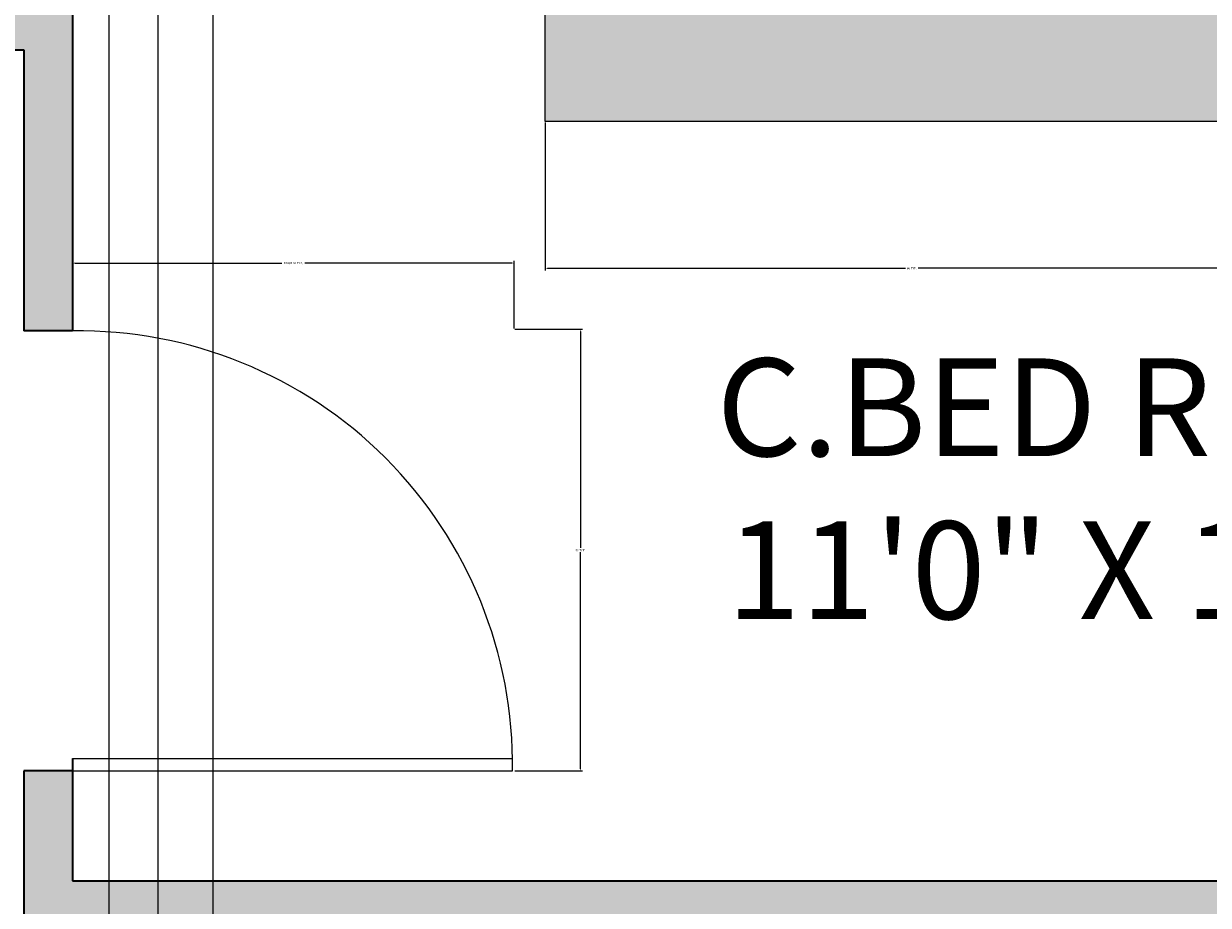
# Model space of a CAD drawing. Units: inches. Extents: x 1567 to 1964, y 1813 to 2447.
# Tile 25 of 28: x 1788 to 1885, y 2261 to 2333. Entities that reach past the tile are written whole.
import ezdxf

# ---------------------------------------------------------------- set-up
doc = ezdxf.new("R2010")
doc.units = ezdxf.units.IN
for name, color, linetype, lineweight in [('A-ANNO-DIMS', 2, 'Continuous', 18), ('A-AREA-IDEN', 7, 'Continuous', 18), ('A-DOOR', 4, 'Continuous', 18), ('A-FURN', 8, 'Continuous', 18), ('A-WALL', 7, 'Continuous', 35)]:
    doc.layers.add(name, color=color, linetype=linetype, lineweight=lineweight)
doc.layers.add('A-FURN-PATT', color=252, linetype='Continuous', lineweight=13, true_color=0x939598)
doc.layers.add('A-WALL-PATT', color=251, linetype='Continuous', lineweight=13, true_color=0x636466)
doc.styles.get("Standard").update_dxf_attribs({"font": 'arial.ttf'})
doc.dimstyles.get("Standard").update_dxf_attribs({"dimtxt": 0.18, "dimasz": 0.18, "dimexe": 0.18, "dimexo": 0.0625, "dimgap": 0.09, "dimtad": 0, "dimtih": 1, "dimtoh": 1, "dimdec": 4, "dimzin": 0, "dimdsep": 46, "dimtxsty": 'Standard', "dimcen": 0.09, "dimadec": 0, "dimazin": 0, "dimtfac": 1, "dimtdec": 4, "dimtofl": 0, "dimtmove": 0, "dimatfit": 3, "dimfxl": 1, "dimtolj": 1, "dimtzin": 0, "dimarcsym": 0})

# ---------------------------------------------------------------- blocks, each defined once
blk = doc.blocks.new('Bed - Queen')
for p, q in [((0, -80.00003), (0, 0)), ((59.99999, -80.00003), (0, -80.00003))]:
    blk.add_line(p, q)
blk = doc.blocks.new('DOOR-SWING-36IN')
for p, q in [((0, 36.001), (0, 0.001)), ((1, 36.001), (1, 0.001))]:
    blk.add_line(p, q)
blk.add_arc((0.5, 35.501), 35.504, 269.19307, 0.80693)
blk = doc.blocks.new('*D16')
at = {"layer": 'A-ANNO-DIMS', "color": 0, "lineweight": -2, "transparency": 16777216}
for p, q in [((1831.109, 2325.358), (1831.109, 2313.24)), ((1891.109, 2325.358), (1891.109, 2313.24)), ((1831.289, 2313.42), (1860.581, 2313.42)), ((1890.929, 2313.42), (1861.638, 2313.42))]:
    blk.add_line(p, q, dxfattribs=at)
at = {"layer": 'A-ANNO-DIMS', "color": 0, "transparency": 16777216}
for points in [[(1831.289, 2313.45), (1831.289, 2313.39), (1831.109, 2313.42)], [(1890.929, 2313.45), (1890.929, 2313.39), (1891.109, 2313.42)]]:
    blk.add_solid(points, dxfattribs=at)
at = {"layer": 'Defpoints', "color": 0, "transparency": 16777216}
for p in [(1831.109, 2325.42), (1891.109, 2325.42), (1891.109, 2313.42)]:
    blk.add_point(p, dxfattribs=at)
at = {"layer": 'A-ANNO-DIMS', "color": 0, "transparency": 16777216, "insert": (1861.109, 2313.42), "char_height": 0.18, "attachment_point": 5}
blk.add_mtext('\\A1;60 TYP.', dxfattribs=at)
blk = doc.blocks.new('*D29')
at = {"layer": 'A-ANNO-DIMS', "color": 0, "lineweight": -2, "transparency": 16777216}
for p, q in [((1792.43, 2308.488), (1792.43, 2314.025)), ((1828.565, 2308.488), (1828.565, 2314.025)), ((1792.61, 2313.845), (1809.561, 2313.845)), ((1828.385, 2313.845), (1811.433, 2313.845))]:
    blk.add_line(p, q, dxfattribs=at)
at = {"layer": 'A-ANNO-DIMS', "color": 0, "transparency": 16777216}
for points in [[(1792.61, 2313.875), (1792.61, 2313.815), (1792.43, 2313.845)], [(1828.385, 2313.875), (1828.385, 2313.815), (1828.565, 2313.845)]]:
    blk.add_solid(points, dxfattribs=at)
at = {"layer": 'Defpoints', "color": 0, "transparency": 16777216}
for p in [(1792.43, 2313.845), (1792.43, 2308.425), (1828.565, 2308.425)]:
    blk.add_point(p, dxfattribs=at)
at = {"layer": 'A-ANNO-DIMS', "color": 0, "transparency": 16777216, "insert": (1810.497, 2313.845), "char_height": 0.18, "attachment_point": 5}
blk.add_mtext('\\A1;DOOR 36 TYP.', dxfattribs=at)
blk = doc.blocks.new('*D30')
at = {"layer": 'A-ANNO-DIMS', "color": 0, "lineweight": -2, "transparency": 16777216}
for p, q in [((1828.627, 2308.425), (1834.165, 2308.425)), ((1833.985, 2308.245), (1833.985, 2290.539)), ((1833.985, 2272.47), (1833.985, 2290.176)), ((1828.627, 2272.29), (1834.165, 2272.29))]:
    blk.add_line(p, q, dxfattribs=at)
at = {"layer": 'A-ANNO-DIMS', "color": 0, "transparency": 16777216}
for points in [[(1833.955, 2308.245), (1834.015, 2308.245), (1833.985, 2308.425)], [(1833.955, 2272.47), (1834.015, 2272.47), (1833.985, 2272.29)]]:
    blk.add_solid(points, dxfattribs=at)
at = {"layer": 'Defpoints', "color": 0, "transparency": 16777216}
for p in [(1828.565, 2308.425), (1833.985, 2308.425), (1828.565, 2272.29)]:
    blk.add_point(p, dxfattribs=at)
at = {"layer": 'A-ANNO-DIMS', "color": 0, "transparency": 16777216, "insert": (1833.985, 2290.358), "char_height": 0.18, "attachment_point": 5}
blk.add_mtext('\\A1;36 TYP.', dxfattribs=at)
blk = doc.blocks.new('*D54')
at = {"layer": 'A-ANNO-DIMS', "color": 0, "lineweight": -2, "transparency": 16777216}
for p, q in [((1711.43, 1964.352), (1711.43, 2447.12)), ((1711.61, 2446.94), (1753.211, 2446.94)), ((1795.25, 2446.94), (1753.648, 2446.94)), ((1795.43, 1964.352), (1795.43, 2447.12))]:
    blk.add_line(p, q, dxfattribs=at)
at = {"layer": 'A-ANNO-DIMS', "color": 0, "transparency": 16777216}
for points in [[(1711.61, 2446.97), (1711.61, 2446.91), (1711.43, 2446.94)], [(1795.25, 2446.97), (1795.25, 2446.91), (1795.43, 2446.94)]]:
    blk.add_solid(points, dxfattribs=at)
at = {"layer": 'Defpoints', "color": 0, "transparency": 16777216}
for p in [(1795.43, 2446.94), (1711.43, 1964.29), (1795.43, 1964.29)]:
    blk.add_point(p, dxfattribs=at)
at = {"layer": 'A-ANNO-DIMS', "color": 0, "transparency": 16777216, "insert": (1753.43, 2446.94), "char_height": 0.18, "attachment_point": 5}
blk.add_mtext('\\A1;84', dxfattribs=at)
blk = doc.blocks.new('*D55')
at = {"layer": 'A-ANNO-DIMS', "color": 0, "lineweight": -2, "transparency": 16777216}
for p, q in [((1795.43, 1964.352), (1795.43, 2447.12)), ((1795.61, 2446.94), (1797.277, 2446.94)), ((1799.25, 2446.94), (1797.582, 2446.94)), ((1799.43, 1967.352), (1799.43, 2447.12))]:
    blk.add_line(p, q, dxfattribs=at)
at = {"layer": 'A-ANNO-DIMS', "color": 0, "transparency": 16777216}
for points in [[(1795.61, 2446.97), (1795.61, 2446.91), (1795.43, 2446.94)], [(1799.25, 2446.97), (1799.25, 2446.91), (1799.43, 2446.94)]]:
    blk.add_solid(points, dxfattribs=at)
at = {"layer": 'Defpoints', "color": 0, "transparency": 16777216}
for p in [(1799.43, 2446.94), (1799.43, 1967.29), (1795.43, 1964.29)]:
    blk.add_point(p, dxfattribs=at)
at = {"layer": 'A-ANNO-DIMS', "color": 0, "transparency": 16777216, "insert": (1797.43, 2446.94), "char_height": 0.18, "attachment_point": 5}
blk.add_mtext('\\A1;4', dxfattribs=at)
blk = doc.blocks.new('*D70')
at = {"layer": 'A-ANNO-DIMS', "color": 0, "lineweight": -2, "transparency": 16777216}
for p, q in [((1799.43, 1967.352), (1799.43, 2447.12)), ((1799.61, 2446.94), (1801.421, 2446.94)), ((1803.75, 2446.94), (1801.938, 2446.94)), ((1803.93, 1967.352), (1803.93, 2447.12))]:
    blk.add_line(p, q, dxfattribs=at)
at = {"layer": 'A-ANNO-DIMS', "color": 0, "transparency": 16777216}
for points in [[(1799.61, 2446.97), (1799.61, 2446.91), (1799.43, 2446.94)], [(1803.75, 2446.97), (1803.75, 2446.91), (1803.93, 2446.94)]]:
    blk.add_solid(points, dxfattribs=at)
at = {"layer": 'Defpoints', "color": 0, "transparency": 16777216}
for p in [(1803.93, 2446.94), (1799.43, 1967.29), (1803.93, 1967.29)]:
    blk.add_point(p, dxfattribs=at)
at = {"layer": 'A-ANNO-DIMS', "color": 0, "transparency": 16777216, "insert": (1801.68, 2446.94), "char_height": 0.18, "attachment_point": 5}
blk.add_mtext('\\A1;4.5', dxfattribs=at)
blk = doc.blocks.new('*D71')
at = {"layer": 'A-ANNO-DIMS', "color": 0, "lineweight": -2, "transparency": 16777216}
for p, q in [((1799.43, 1910.752), (1799.43, 2447.12)), ((1799.61, 2446.94), (1861.648, 2446.94)), ((1924.25, 2446.94), (1862.211, 2446.94)), ((1924.43, 1910.752), (1924.43, 2447.12))]:
    blk.add_line(p, q, dxfattribs=at)
at = {"layer": 'A-ANNO-DIMS', "color": 0, "transparency": 16777216}
for points in [[(1799.61, 2446.97), (1799.61, 2446.91), (1799.43, 2446.94)], [(1924.25, 2446.97), (1924.25, 2446.91), (1924.43, 2446.94)]]:
    blk.add_solid(points, dxfattribs=at)
at = {"layer": 'Defpoints', "color": 0, "transparency": 16777216}
for p in [(1924.43, 2446.94), (1799.43, 1910.69), (1924.43, 1910.69)]:
    blk.add_point(p, dxfattribs=at)
at = {"layer": 'A-ANNO-DIMS', "color": 0, "transparency": 16777216, "insert": (1861.93, 2446.94), "char_height": 0.18, "attachment_point": 5}
blk.add_mtext('\\A1;125', dxfattribs=at)

msp = doc.modelspace()

# ---------------------------------------------------------------- hatches: boundary and pattern name
at = {"layer": 'A-FURN-PATT'}
h = msp.add_hatch(color=256, dxfattribs=at)
h.dxf.hatch_style = 1
h.paths.add_polyline_path([(1697.3402, 2374.8316), (1682.1402, 2374.8316), (1682.1402, 2387.6316), (1637.3402, 2387.6316), (1637.3402, 2324.4315), (1697.3402, 2324.4315)])
h.paths.add_polyline_path([(1891.1093, 2375.8204), (1875.9094, 2375.8204), (1875.9094, 2388.6204), (1831.1094, 2388.6204), (1831.1094, 2325.4204), (1891.1093, 2325.4204)])
h.paths.add_polyline_path([(1702.5611, 2206.8057), (1702.5611, 2210.8057), (1699.7395, 2209.9436), (1697.013, 2209.2403), (1694.3857, 2208.6763), (1691.8615, 2208.2326), (1689.4443, 2207.8896), (1687.1381, 2207.6282), (1684.9469, 2207.4289), (1682.8747, 2207.2725), (1680.9233, 2207.1425), (1679.0865, 2207.0339), (1677.3558, 2206.9445), (1675.7229, 2206.8719), (1674.1794, 2206.8141), (1672.7169, 2206.7688), (1671.327, 2206.7339), (1670.0014, 2206.707), (1668.7314, 2206.6866), (1667.5072, 2206.6732), (1666.3188, 2206.668), (1665.1561, 2206.6722), (1664.009, 2206.6869), (1662.8675, 2206.7133), (1661.7215, 2206.7525), (1660.5611, 2206.8057), (1660.5611, 2202.8057), (1661.9932, 2202.9556), (1663.3314, 2203.0744), (1664.5899, 2203.1671), (1665.7831, 2203.2385), (1666.9254, 2203.2935), (1668.0311, 2203.3368), (1669.1145, 2203.3734), (1670.1902, 2203.4081), (1671.2724, 2203.4451), (1672.3759, 2203.4866), (1673.5155, 2203.534), (1674.706, 2203.5887), (1675.9621, 2203.6523), (1677.2986, 2203.7262), (1678.7304, 2203.8118), (1680.2722, 2203.9108), (1681.947, 2204.0272), (1683.8108, 2204.1769), (1685.9279, 2204.3782), (1688.3626, 2204.6496), (1691.179, 2205.0096), (1694.4413, 2205.4767), (1698.214, 2206.0692)])
h.paths.add_polyline_path([(1702.5611, 2218.8057), (1701.9821, 2217.9383), (1701.3316, 2217.191), (1700.6091, 2216.5515), (1699.8141, 2216.0071), (1698.946, 2215.5454), (1698.0041, 2215.1536), (1696.9879, 2214.8194), (1695.8969, 2214.5301), (1694.7328, 2214.2753), (1693.5072, 2214.0522), (1692.2339, 2213.8602), (1690.9266, 2213.6989), (1689.5994, 2213.5675), (1688.266, 2213.4654), (1686.9402, 2213.392), (1685.636, 2213.3467), (1684.3619, 2213.3287), (1683.1053, 2213.3361), (1681.8482, 2213.3668), (1680.5727, 2213.4187), (1679.2608, 2213.4898), (1677.8948, 2213.5779), (1676.4565, 2213.6811), (1674.9282, 2213.7971), (1673.2982, 2213.9236), (1671.5804, 2214.0573), (1669.795, 2214.1945), (1667.9622, 2214.3316), (1666.1022, 2214.4649), (1664.2352, 2214.5908), (1662.3814, 2214.7056), (1660.5611, 2214.8057), (1660.5611, 2206.8057), (1661.7215, 2206.7525), (1662.8675, 2206.7133), (1664.009, 2206.6869), (1665.1561, 2206.6722), (1666.3188, 2206.668), (1667.5072, 2206.6732), (1668.7314, 2206.6866), (1670.0014, 2206.707), (1671.327, 2206.7339), (1672.7169, 2206.7688), (1674.1794, 2206.8141), (1675.7229, 2206.8719), (1677.3558, 2206.9445), (1679.0865, 2207.0339), (1680.9233, 2207.1425), (1682.8747, 2207.2725), (1684.9469, 2207.4289), (1687.1381, 2207.6282), (1689.4443, 2207.8896), (1691.8615, 2208.2326), (1694.3857, 2208.6763), (1697.013, 2209.2403), (1699.7395, 2209.9436), (1702.5611, 2210.8057)])
h.paths.add_polyline_path([(1700.6091, 2216.5515), (1701.3316, 2217.191), (1701.9821, 2217.9383), (1702.5611, 2218.8057), (1702.5611, 2222.8057), (1689.452, 2222.8057), (1689.0171, 2222.4556), (1688.4521, 2222.0354), (1687.7806, 2221.5662), (1687.0235, 2221.067), (1686.2019, 2220.5566), (1685.3367, 2220.0541), (1684.4491, 2219.5785), (1683.56, 2219.1486), (1682.6867, 2218.7795), (1681.8312, 2218.4692), (1680.9918, 2218.212), (1680.1667, 2218.0019), (1679.3541, 2217.833), (1678.5524, 2217.6995), (1677.7597, 2217.5954), (1676.9744, 2217.5149), (1676.1942, 2217.4531), (1675.4146, 2217.4093), (1674.6309, 2217.384), (1673.8381, 2217.3774), (1673.0313, 2217.39), (1672.2056, 2217.4221), (1671.3562, 2217.4741), (1670.4782, 2217.5463), (1669.5642, 2217.639), (1668.5968, 2217.7516), (1667.5562, 2217.8833), (1666.4226, 2218.0336), (1665.1761, 2218.2017), (1663.7969, 2218.3869), (1662.2651, 2218.5885), (1660.5611, 2218.8057), (1660.5611, 2214.8057), (1662.3814, 2214.7056), (1664.2352, 2214.5908), (1666.1022, 2214.4649), (1667.9622, 2214.3316), (1669.795, 2214.1945), (1671.5804, 2214.0573), (1673.2982, 2213.9236), (1674.9282, 2213.7971), (1676.4565, 2213.6811), (1677.8948, 2213.5779), (1679.2608, 2213.4898), (1680.5727, 2213.4187), (1681.8482, 2213.3668), (1683.1053, 2213.3361), (1684.3619, 2213.3287), (1685.636, 2213.3467), (1686.9402, 2213.392), (1688.266, 2213.4654), (1689.5994, 2213.5675), (1690.9266, 2213.6989), (1692.2339, 2213.8602), (1693.5072, 2214.0522), (1694.7328, 2214.2753), (1695.8969, 2214.5301), (1696.9879, 2214.8194), (1698.0041, 2215.1536), (1698.946, 2215.5454), (1699.8141, 2216.0071)])
h.paths.add_polyline_path([(1687.0235, 2221.067), (1687.7806, 2221.5662), (1688.4521, 2222.0354), (1689.0171, 2222.4556), (1689.452, 2222.8057), (1660.5611, 2222.8057), (1660.5611, 2218.8057), (1662.2651, 2218.5885), (1663.7969, 2218.3869), (1665.1761, 2218.2017), (1666.4226, 2218.0336), (1667.5562, 2217.8833), (1668.5968, 2217.7516), (1669.5642, 2217.639), (1670.4782, 2217.5463), (1671.3562, 2217.4741), (1672.2056, 2217.4221), (1673.0313, 2217.39), (1673.8381, 2217.3774), (1674.6309, 2217.384), (1675.4146, 2217.4093), (1676.1942, 2217.4531), (1676.9744, 2217.5149), (1677.7597, 2217.5954), (1678.5524, 2217.6995), (1679.3541, 2217.833), (1680.1667, 2218.0019), (1680.9918, 2218.212), (1681.8312, 2218.4692), (1682.6867, 2218.7795), (1683.56, 2219.1486), (1684.4491, 2219.5785), (1685.3367, 2220.0541), (1686.2019, 2220.5566)], flags=17)
h.paths.add_polyline_path([(1702.5611, 2198.8057), (1698.9289, 2199.2412), (1695.8472, 2199.5774), (1693.2166, 2199.8257), (1690.9377, 2199.9973), (1688.9111, 2200.1033), (1687.0375, 2200.155), (1685.2174, 2200.1637), (1683.3514, 2200.1406), (1681.3514, 2200.0941), (1679.1736, 2200.0225), (1676.7858, 2199.921), (1674.1554, 2199.7852), (1671.2502, 2199.6103), (1668.0377, 2199.3919), (1664.4854, 2199.1252), (1660.5611, 2198.8057), (1660.5611, 2194.8057), (1662.2697, 2194.9771), (1663.9673, 2195.0999), (1665.6339, 2195.1809), (1667.2495, 2195.227), (1668.7941, 2195.2449), (1670.2478, 2195.2414), (1671.5906, 2195.2233), (1672.8026, 2195.1974), (1673.8739, 2195.1689), (1674.8359, 2195.1364), (1675.7302, 2195.0967), (1676.5982, 2195.0469), (1677.4817, 2194.9838), (1678.422, 2194.9043), (1679.4609, 2194.8055), (1680.6397, 2194.6842), (1682.005, 2194.5341), (1683.6223, 2194.335), (1685.562, 2194.0637), (1687.8945, 2193.6967), (1690.6902, 2193.2108), (1694.0196, 2192.5826), (1697.9531, 2191.7887), (1702.5611, 2190.8057)])
h.paths.add_polyline_path([(1702.5611, 2206.8057), (1698.214, 2206.0692), (1694.4413, 2205.4767), (1691.179, 2205.0096), (1688.3626, 2204.6496), (1685.9279, 2204.3782), (1683.8108, 2204.1769), (1681.947, 2204.0272), (1680.2722, 2203.9108), (1678.7304, 2203.8118), (1677.2986, 2203.7262), (1675.9621, 2203.6523), (1674.706, 2203.5887), (1673.5155, 2203.534), (1672.3759, 2203.4866), (1671.2724, 2203.4451), (1670.1902, 2203.4081), (1669.1145, 2203.3734), (1668.0311, 2203.3368), (1666.9254, 2203.2935), (1665.7831, 2203.2385), (1664.5899, 2203.1671), (1663.3314, 2203.0744), (1661.9932, 2202.9556), (1660.5611, 2202.8057), (1660.5611, 2198.8057), (1664.4854, 2199.1252), (1668.0377, 2199.3919), (1671.2502, 2199.6103), (1674.1554, 2199.7852), (1676.7858, 2199.921), (1679.1736, 2200.0225), (1681.3514, 2200.0941), (1683.3514, 2200.1406), (1685.2174, 2200.1637), (1687.0375, 2200.155), (1688.9111, 2200.1033), (1690.9377, 2199.9973), (1693.2166, 2199.8257), (1695.8472, 2199.5774), (1698.9289, 2199.2412), (1702.5611, 2198.8057)])
h.paths.add_polyline_path([(1702.5611, 2190.8057), (1697.9531, 2191.7887), (1694.0196, 2192.5826), (1690.6902, 2193.2108), (1687.8945, 2193.6967), (1685.562, 2194.0637), (1683.6223, 2194.335), (1682.005, 2194.5341), (1680.6397, 2194.6842), (1679.4609, 2194.8055), (1678.422, 2194.9043), (1677.4817, 2194.9838), (1676.5982, 2195.0469), (1675.7302, 2195.0967), (1674.8359, 2195.1364), (1673.8739, 2195.1689), (1672.8026, 2195.1974), (1671.5906, 2195.2233), (1670.2478, 2195.2414), (1668.7941, 2195.2449), (1667.2495, 2195.227), (1665.6339, 2195.1809), (1663.9673, 2195.0999), (1662.2697, 2194.9771), (1660.5611, 2194.8057), (1660.5611, 2190.8057), (1665.9637, 2190.2699), (1670.5105, 2189.7867), (1674.3035, 2189.3504), (1677.4445, 2188.9552), (1680.0354, 2188.5951), (1682.1782, 2188.2644), (1683.9747, 2187.9571), (1685.5268, 2187.6675), (1686.9225, 2187.3901), (1688.1943, 2187.1216), (1689.3606, 2186.859), (1690.4399, 2186.5993), (1691.4508, 2186.3396), (1692.4118, 2186.0769), (1693.3413, 2185.8084), (1694.2579, 2185.531), (1695.1786, 2185.2422), (1696.1142, 2184.9406), (1697.0739, 2184.6252), (1698.0671, 2184.2949), (1699.1032, 2183.9489), (1700.1913, 2183.586), (1701.3408, 2183.2053), (1702.5611, 2182.8057)])
h.paths.add_polyline_path([(1702.5611, 2182.8057), (1701.3408, 2183.2053), (1700.1913, 2183.586), (1699.1032, 2183.9489), (1698.0671, 2184.2949), (1697.0739, 2184.6252), (1696.1142, 2184.9406), (1695.1786, 2185.2422), (1694.2579, 2185.531), (1693.3413, 2185.8084), (1692.4118, 2186.0769), (1691.4508, 2186.3396), (1690.4399, 2186.5993), (1689.3606, 2186.859), (1688.1943, 2187.1216), (1686.9225, 2187.3901), (1685.5268, 2187.6675), (1683.9747, 2187.9571), (1682.1782, 2188.2644), (1680.0354, 2188.5951), (1677.4445, 2188.9552), (1674.3035, 2189.3504), (1670.5105, 2189.7867), (1665.9637, 2190.2699), (1660.5611, 2190.8057), (1660.5611, 2186.8057), (1663.5709, 2186.52), (1666.0965, 2186.2414), (1668.1979, 2185.9698), (1669.9351, 2185.7048), (1671.3681, 2185.446), (1672.5568, 2185.1931), (1673.5613, 2184.9458), (1674.4415, 2184.7037), (1675.2485, 2184.4664), (1675.9976, 2184.2328), (1677.0295, 2183.8907), (1678.2492, 2183.4332), (1679.354, 2182.9669), (1680.4123, 2182.4724), (1681.3757, 2181.9718), (1682.2435, 2181.4594), (1683.1864, 2180.8057), (1702.5611, 2180.8057)])
h.paths.add_polyline_path([(1677.3469, 2183.7716), (1676.6949, 2184.0016), (1675.9976, 2184.2328), (1675.2485, 2184.4664), (1674.4415, 2184.7037), (1673.5613, 2184.9458), (1672.5568, 2185.1931), (1671.3681, 2185.446), (1669.9351, 2185.7048), (1668.1979, 2185.9698), (1666.0965, 2186.2414), (1663.5709, 2186.52), (1660.5611, 2186.8057), (1660.5611, 2180.8057), (1683.1506, 2180.8057), (1682.802, 2181.0722), (1682.4264, 2181.3326), (1682.0201, 2181.5913), (1681.586, 2181.8476), (1681.1268, 2182.1011), (1680.6453, 2182.3513), (1680.1443, 2182.5976), (1679.6266, 2182.8395), (1679.0933, 2183.0769), (1678.5398, 2183.3105), (1677.9598, 2183.5417)], flags=17)
h.paths.add_polyline_path([(1824.4511, 2199.9016), (1824.089, 2199.9302), (1824.0595, 2199.9372), (1824.0397, 2199.9406), (1823.5413, 2200.0576), (1823.4095, 2200.0864), (1823.0664, 2200.1559), (1822.6419, 2200.2361), (1822.1519, 2200.3222), (1821.6126, 2200.4093), (1821.0401, 2200.4925), (1820.4505, 2200.5669), (1819.8599, 2200.6276), (1819.2845, 2200.6697), (1818.7366, 2200.6896), (1818.2141, 2200.688), (1817.7112, 2200.6668), (1817.222, 2200.6281), (1816.7405, 2200.5737), (1816.261, 2200.5057), (1815.7776, 2200.4259), (1815.2845, 2200.3364), (1814.3007, 2200.149), (1813.3315, 2199.9765), (1812.406, 2199.8514), (1811.6868, 2199.7739), (1810.8992, 2199.7121), (1810.0345, 2199.6697), (1809.0854, 2199.6497), (1808.0514, 2199.6502), (1806.9334, 2199.6683), (1805.7324, 2199.701), (1804.4493, 2199.7454), (1803.0852, 2199.7986), (1801.641, 2199.8577), (1800.1178, 2199.9197), (1798.5134, 2199.9818), (1796.8144, 2200.0415), (1795.004, 2200.0962), (1793.0657, 2200.1437), (1790.9828, 2200.1814), (1788.7389, 2200.2068), (1786.3171, 2200.2177), (1783.7011, 2200.2114), (1780.8715, 2200.185), (1777.7988, 2200.1326), (1774.4506, 2200.0481), (1770.7948, 2199.9249), (1766.7992, 2199.7569), (1762.4316, 2199.5376), (1757.6596, 2199.2606), (1752.4511, 2198.9197), (1752.4511, 2193.4197), (1761.2668, 2193.6071), (1768.3671, 2193.7934), (1773.9821, 2193.9778), (1778.3417, 2194.1593), (1781.6759, 2194.3369), (1784.2148, 2194.5096), (1786.1882, 2194.6764), (1787.8261, 2194.8364), (1789.3219, 2194.9887), (1790.7226, 2195.1333), (1792.0383, 2195.27), (1793.2792, 2195.3989), (1794.4557, 2195.52), (1795.5781, 2195.6333), (1796.6564, 2195.7387), (1797.7011, 2195.8364), (1798.7216, 2195.9259), (1799.7245, 2196.0057), (1800.7158, 2196.0737), (1801.7011, 2196.1281), (1802.6865, 2196.1668), (1803.6777, 2196.188), (1804.6806, 2196.1896), (1805.7011, 2196.1697), (1806.7423, 2196.1273), (1807.7962, 2196.0643), (1808.852, 2195.9837), (1809.899, 2195.8885), (1810.9265, 2195.7815), (1811.9238, 2195.6658), (1812.88, 2195.5442), (1813.7845, 2195.4197), (1814.6296, 2195.2948), (1815.4205, 2195.1704), (1816.1656, 2195.0469), (1816.873, 2194.9249), (1817.5511, 2194.8049), (1818.2083, 2194.6873), (1818.8527, 2194.5726), (1819.4928, 2194.4614), (1820.1348, 2194.3554), (1820.7773, 2194.2615), (1821.4169, 2194.1882), (1822.0501, 2194.1437), (1822.6735, 2194.1363), (1823.2838, 2194.1743), (1823.8775, 2194.266), (1824.4511, 2194.4197)])
h.paths.add_polyline_path([(1821.4716, 2190.5098), (1820.4303, 2190.5708), (1819.3811, 2190.6415), (1818.3339, 2190.7186), (1817.2985, 2190.7986), (1816.2845, 2190.8781), (1815.2976, 2190.9542), (1814.3274, 2191.0259), (1813.3592, 2191.0927), (1812.3782, 2191.1541), (1811.3699, 2191.2097), (1810.3196, 2191.2589), (1809.2127, 2191.3013), (1808.0345, 2191.3364), (1806.7708, 2191.3634), (1805.4094, 2191.3807), (1803.9387, 2191.3862), (1802.3469, 2191.3781), (1800.6223, 2191.3543), (1798.7532, 2191.313), (1796.7278, 2191.2521), (1794.5344, 2191.1697), (1792.128, 2191.0648), (1789.33, 2190.9393), (1785.9285, 2190.7962), (1781.7115, 2190.6385), (1776.4672, 2190.469), (1769.9836, 2190.2908), (1762.0489, 2190.1067), (1752.4511, 2189.9197), (1752.4511, 2185.4197), (1758.363, 2185.5846), (1763.4179, 2185.7075), (1767.7199, 2185.7933), (1771.373, 2185.8468), (1774.4811, 2185.873), (1777.1484, 2185.8768), (1779.4787, 2185.8629), (1781.5761, 2185.8364), (1783.5287, 2185.8014), (1785.3606, 2185.7596), (1787.0802, 2185.7119), (1788.6959, 2185.6593), (1790.2158, 2185.6028), (1791.6484, 2185.5434), (1793.0018, 2185.4821), (1794.2844, 2185.4197), (1795.5065, 2185.3576), (1796.6861, 2185.298), (1797.8433, 2185.2432), (1798.998, 2185.1958), (1800.1703, 2185.1581), (1801.3801, 2185.1326), (1802.6476, 2185.1218), (1803.9928, 2185.1281), (1805.4444, 2185.1555), (1807.0663, 2185.2147), (1808.9315, 2185.3178), (1811.1126, 2185.477), (1813.6823, 2185.7046), (1816.7135, 2186.0128), (1820.2788, 2186.4138), (1824.4511, 2186.9197), (1824.4511, 2190.4197), (1823.4918, 2190.4309), (1822.4954, 2190.4621)])
h.paths.add_polyline_path([(1797.3762, 2216.0584), (1797.6199, 2216.2267), (1797.9558, 2216.3355), (1798.3017, 2216.3703), (1798.5761, 2216.3781), (1798.8974, 2216.3703), (1799.2714, 2216.3468), (1799.704, 2216.3078), (1800.2011, 2216.2531), (1800.7695, 2216.1829), (1801.4205, 2216.0981), (1802.1662, 2215.9996), (1803.0188, 2215.8885), (1803.9906, 2215.7656), (1805.0937, 2215.632), (1806.3404, 2215.4886), (1807.7428, 2215.3364), (1809.3101, 2215.1764), (1811.039, 2215.0096), (1812.9232, 2214.8369), (1814.9563, 2214.6593), (1817.132, 2214.4778), (1819.444, 2214.2934), (1821.8858, 2214.1071), (1824.4511, 2213.9197), (1824.4511, 2217.9197), (1752.4511, 2217.9197), (1752.4511, 2214.9197), (1757.2739, 2214.8973), (1761.6432, 2214.8338), (1765.5973, 2214.7352), (1769.1751, 2214.6072), (1772.4149, 2214.4559), (1775.3554, 2214.2869), (1778.0352, 2214.1063), (1780.4928, 2213.9197), (1782.7607, 2213.7329), (1784.8476, 2213.5499), (1786.7557, 2213.3748), (1788.4876, 2213.2114), (1790.0456, 2213.0636), (1791.4322, 2212.9354), (1792.6499, 2212.8305), (1793.7011, 2212.7531), (1794.5904, 2212.7059), (1795.3313, 2212.688), (1795.9394, 2212.6974), (1796.4303, 2212.7322), (1796.8196, 2212.7905), (1797.123, 2212.8703), (1797.356, 2212.9695), (1797.5344, 2213.0864), (1797.6716, 2213.2187), (1797.7727, 2213.3637), (1797.8406, 2213.5185), (1797.8782, 2213.6801), (1797.8884, 2213.8457), (1797.8743, 2214.0122), (1797.8386, 2214.1767), (1797.7844, 2214.3364), (1797.7149, 2214.4889), (1797.6347, 2214.6346), (1797.5486, 2214.7744), (1797.3327, 2215.109), (1797.178, 2215.4303), (1797.1896, 2215.7939)])
h.paths.add_polyline_path([(1804.7872, 2210.6789), (1804.546, 2211.022), (1804.3512, 2211.3917), (1804.2466, 2211.7546), (1804.2574, 2212.0998), (1804.4058, 2212.4178), (1804.7068, 2212.7007), (1805.1359, 2212.9124), (1805.5279, 2212.9926), (1805.8136, 2213.0154), (1806.1178, 2213.0031), (1806.4405, 2212.9529), (1806.7929, 2212.867), (1807.1893, 2212.7489), (1807.6438, 2212.602), (1808.1706, 2212.4297), (1808.7838, 2212.2355), (1809.4976, 2212.0227), (1810.3261, 2211.7947), (1811.2868, 2211.5533), (1812.4101, 2211.2928), (1813.7297, 2211.0059), (1815.2793, 2210.6854), (1817.0925, 2210.3238), (1819.2031, 2209.9139), (1821.6447, 2209.4483), (1824.4511, 2208.9197), (1824.4511, 2213.9197), (1821.8858, 2214.1071), (1819.444, 2214.2934), (1817.132, 2214.4778), (1814.9563, 2214.6593), (1812.9232, 2214.8369), (1811.039, 2215.0096), (1809.3101, 2215.1764), (1807.7428, 2215.3364), (1806.3404, 2215.4886), (1805.0937, 2215.632), (1803.9906, 2215.7656), (1803.0188, 2215.8885), (1802.1662, 2215.9996), (1801.4205, 2216.0981), (1800.7695, 2216.1829), (1800.2011, 2216.2531), (1799.704, 2216.3078), (1799.2714, 2216.3468), (1798.8974, 2216.3703), (1798.5761, 2216.3781), (1798.3017, 2216.3703), (1798.0683, 2216.3468), (1797.87, 2216.3078), (1797.7011, 2216.2531), (1797.5566, 2216.1831), (1797.4355, 2216.0994), (1797.3378, 2216.004), (1797.2636, 2215.8989), (1797.2128, 2215.7859), (1797.1855, 2215.6671), (1797.1816, 2215.5444), (1797.2011, 2215.4197), (1797.2433, 2215.2946), (1797.304, 2215.1684), (1797.3783, 2215.0403), (1797.4615, 2214.9093), (1797.6718, 2214.5836), (1797.8218, 2214.2545), (1797.8933, 2213.9247), (1797.8728, 2213.5918), (1797.7366, 2213.2814), (1797.4586, 2213.0132), (1797.123, 2212.8703), (1796.8196, 2212.7905), (1796.4303, 2212.7322), (1795.9394, 2212.6974), (1795.3313, 2212.688), (1794.5904, 2212.7059), (1793.7011, 2212.7531), (1792.6499, 2212.8305), (1791.4322, 2212.9354), (1790.0456, 2213.0636), (1788.4876, 2213.2114), (1786.7557, 2213.3748), (1784.8476, 2213.5499), (1782.7607, 2213.7329), (1780.4928, 2213.9197), (1778.0352, 2214.1063), (1775.3554, 2214.2869), (1772.4149, 2214.4559), (1769.1751, 2214.6072), (1765.5973, 2214.7352), (1761.6432, 2214.8338), (1757.2739, 2214.8973), (1752.4511, 2214.9197), (1752.4511, 2209.9197), (1759.4745, 2210.0625), (1765.2786, 2210.1242), (1770.027, 2210.1175), (1773.8834, 2210.0551), (1777.0112, 2209.9498), (1779.5741, 2209.8143), (1781.7357, 2209.6611), (1783.6594, 2209.5031), (1785.4813, 2209.3506), (1787.2265, 2209.2049), (1788.8926, 2209.0651), (1790.4771, 2208.9301), (1791.9777, 2208.7991), (1793.3919, 2208.671), (1794.7171, 2208.5449), (1795.9511, 2208.4197), (1797.0922, 2208.2952), (1798.1425, 2208.1736), (1799.1049, 2208.0579), (1799.9823, 2207.951), (1800.7778, 2207.8558), (1801.4941, 2207.7752), (1802.1342, 2207.7122), (1802.7011, 2207.6697), (1803.1982, 2207.65), (1803.6308, 2207.6528), (1804.0048, 2207.6771), (1804.3261, 2207.7218), (1804.6005, 2207.7861), (1804.8339, 2207.869), (1805.0322, 2207.9694), (1805.2011, 2208.0864), (1805.3455, 2208.2189), (1805.4654, 2208.365), (1805.56, 2208.5229), (1805.6282, 2208.6906), (1805.6691, 2208.866), (1805.6816, 2209.0473), (1805.6648, 2209.2326), (1805.6178, 2209.4197), (1805.5406, 2209.6072), (1805.4381, 2209.7947), (1805.316, 2209.9822), (1805.1803, 2210.1697), (1805.0367, 2210.3572)])
h.paths.add_polyline_path([(1801.4941, 2207.7752), (1800.7778, 2207.8558), (1799.9823, 2207.951), (1799.1049, 2208.0579), (1798.1425, 2208.1736), (1797.0922, 2208.2952), (1795.9511, 2208.4197), (1794.7171, 2208.5449), (1793.3919, 2208.671), (1791.9777, 2208.7991), (1790.4771, 2208.9301), (1788.8926, 2209.0651), (1787.2265, 2209.2049), (1785.4813, 2209.3506), (1783.6594, 2209.5031), (1781.7357, 2209.6611), (1779.5741, 2209.8143), (1777.0112, 2209.9498), (1773.8834, 2210.0551), (1770.027, 2210.1175), (1765.2786, 2210.1242), (1759.4745, 2210.0625), (1752.4511, 2209.9197), (1752.4511, 2205.4197), (1757.7354, 2205.2545), (1762.3821, 2205.1294), (1766.4565, 2205.0374), (1770.024, 2204.9718), (1773.1502, 2204.9258), (1775.9003, 2204.8924), (1778.3399, 2204.8649), (1780.5344, 2204.8364), (1782.5421, 2204.8014), (1784.3925, 2204.7596), (1786.1082, 2204.7119), (1787.7115, 2204.6593), (1789.225, 2204.6028), (1790.6711, 2204.5434), (1792.0724, 2204.4821), (1793.4511, 2204.4197), (1794.8241, 2204.3576), (1796.1855, 2204.2973), (1797.5234, 2204.241), (1798.8261, 2204.1906), (1800.082, 2204.1479), (1801.2792, 2204.115), (1802.4062, 2204.0939), (1803.4511, 2204.0864), (1804.4051, 2204.0942), (1805.2701, 2204.1176), (1806.0512, 2204.1567), (1806.7532, 2204.2114), (1807.381, 2204.2817), (1807.9394, 2204.3676), (1808.4334, 2204.4692), (1808.8678, 2204.5864), (1809.248, 2204.7187), (1809.5813, 2204.8637), (1809.8756, 2205.0185), (1810.1386, 2205.1801), (1810.3782, 2205.3457), (1810.6022, 2205.5122), (1810.9725, 2205.7941), (1811.3803, 2206.072), (1811.739, 2206.2612), (1812.0032, 2206.3781), (1812.2869, 2206.4793), (1812.5931, 2206.563), (1812.9246, 2206.6271), (1813.2845, 2206.6697), (1813.6746, 2206.6894), (1814.0931, 2206.6867), (1814.5369, 2206.6624), (1815.0032, 2206.6176), (1815.489, 2206.5534), (1815.9915, 2206.4705), (1816.5076, 2206.3701), (1817.0345, 2206.2531), (1817.5753, 2206.1196), (1818.1582, 2205.9666), (1818.8172, 2205.7902), (1819.5865, 2205.5864), (1820.5004, 2205.3514), (1821.5931, 2205.0812), (1822.8986, 2204.7719), (1824.4511, 2204.4197), (1824.4511, 2208.9197), (1821.6447, 2209.4483), (1819.2031, 2209.9139), (1817.0925, 2210.3238), (1815.2793, 2210.6854), (1813.7297, 2211.0059), (1812.4101, 2211.2928), (1811.2868, 2211.5533), (1810.3261, 2211.7947), (1809.4976, 2212.0227), (1808.7838, 2212.2355), (1808.1706, 2212.4297), (1807.6438, 2212.602), (1807.1893, 2212.7489), (1806.7929, 2212.867), (1806.4405, 2212.9529), (1806.1178, 2213.0031), (1805.8136, 2213.0154), (1805.5279, 2212.9926), (1805.2638, 2212.9386), (1805.024, 2212.8572), (1804.8116, 2212.7524), (1804.6295, 2212.6281), (1804.4806, 2212.4881), (1804.3678, 2212.3364), (1804.2931, 2212.1764), (1804.2545, 2212.0096), (1804.2491, 2211.8369), (1804.274, 2211.6593), (1804.3263, 2211.4778), (1804.4029, 2211.2934), (1804.5011, 2211.1071), (1804.6178, 2210.9197), (1804.7496, 2210.7322), (1804.8912, 2210.5447), (1805.154, 2210.2061), (1805.3962, 2209.8715), (1805.5964, 2209.5053), (1805.688, 2209.1402), (1805.6629, 2208.7758), (1805.5257, 2208.4385), (1805.2839, 2208.1437), (1804.9434, 2207.9078), (1804.6005, 2207.7861), (1804.3261, 2207.7218), (1804.0048, 2207.6771), (1803.6308, 2207.6528), (1803.1982, 2207.65), (1802.7011, 2207.6697), (1802.1342, 2207.7122)])
h.paths.add_polyline_path([(1824.4511, 2204.4197), (1822.8986, 2204.7719), (1821.5931, 2205.0812), (1820.5004, 2205.3514), (1819.5865, 2205.5864), (1818.8172, 2205.7902), (1818.1582, 2205.9666), (1817.5753, 2206.1196), (1817.0345, 2206.2531), (1816.5076, 2206.3701), (1815.9915, 2206.4705), (1815.489, 2206.5534), (1815.0032, 2206.6176), (1814.5369, 2206.6624), (1814.0931, 2206.6867), (1813.6746, 2206.6894), (1813.2845, 2206.6697), (1812.9246, 2206.6271), (1812.5931, 2206.563), (1812.2869, 2206.4793), (1812.0032, 2206.3781), (1811.739, 2206.2612), (1811.4915, 2206.1307), (1811.2576, 2205.9884), (1811.0345, 2205.8364), (1810.8183, 2205.6767), (1810.4357, 2205.3854), (1810.1386, 2205.1801), (1809.8756, 2205.0185), (1809.5813, 2204.8637), (1809.248, 2204.7187), (1808.8678, 2204.5864), (1808.4334, 2204.4692), (1807.9394, 2204.3676), (1807.381, 2204.2817), (1806.7532, 2204.2114), (1806.0512, 2204.1567), (1805.2701, 2204.1176), (1804.4051, 2204.0942), (1803.4511, 2204.0864), (1802.4062, 2204.0939), (1801.2792, 2204.115), (1800.082, 2204.1479), (1798.8261, 2204.1906), (1797.5234, 2204.241), (1796.1855, 2204.2973), (1794.8241, 2204.3576), (1793.4511, 2204.4197), (1792.0724, 2204.4821), (1790.6711, 2204.5434), (1789.225, 2204.6028), (1787.7115, 2204.6593), (1786.1082, 2204.7119), (1784.3925, 2204.7596), (1782.5421, 2204.8014), (1780.5344, 2204.8364), (1778.3399, 2204.8649), (1775.9003, 2204.8924), (1773.1502, 2204.9258), (1770.024, 2204.9718), (1766.4565, 2205.0374), (1762.3821, 2205.1294), (1757.7354, 2205.2545), (1752.4511, 2205.4197), (1752.4511, 2198.9197), (1757.6596, 2199.2606), (1762.4316, 2199.5376), (1766.7992, 2199.7569), (1770.7948, 2199.9249), (1774.4506, 2200.0481), (1777.7988, 2200.1326), (1780.8715, 2200.185), (1783.7011, 2200.2114), (1786.3171, 2200.2177), (1788.7389, 2200.2068), (1790.9828, 2200.1814), (1793.0657, 2200.1437), (1795.004, 2200.0962), (1796.8144, 2200.0415), (1798.5134, 2199.9818), (1800.1178, 2199.9197), (1801.641, 2199.8577), (1803.0852, 2199.7986), (1804.4493, 2199.7454), (1805.7324, 2199.701), (1806.9334, 2199.6683), (1808.0514, 2199.6502), (1809.0854, 2199.6497), (1810.0345, 2199.6697), (1810.8992, 2199.7121), (1811.6868, 2199.7739), (1812.406, 2199.8514), (1813.0657, 2199.9406), (1813.6746, 2200.0376), (1814.2415, 2200.1385), (1814.7752, 2200.2394), (1815.2845, 2200.3364), (1815.7776, 2200.4259), (1816.261, 2200.5057), (1816.7405, 2200.5737), (1817.222, 2200.6281), (1817.7112, 2200.6668), (1818.2141, 2200.688), (1818.7366, 2200.6896), (1819.2845, 2200.6697), (1819.8599, 2200.6276), (1820.4505, 2200.5669), (1821.0401, 2200.4925), (1821.6126, 2200.4093), (1822.1519, 2200.3222), (1822.6419, 2200.2361), (1823.0664, 2200.1559), (1823.5408, 2200.0598), (1824.0595, 2199.9372), (1824.1105, 2199.9285), (1824.1888, 2199.9223), (1824.2953, 2199.9201), (1824.4511, 2199.9197)])
h.paths.add_polyline_path([(1795.4295, 2021.5492), (1771.4295, 2021.5492), (1771.4295, 1988.29), (1735.4295, 1988.29), (1735.4295, 2055.79), (1711.4295, 2055.79), (1711.4295, 1964.29), (1795.4295, 1964.29)])
h.paths.add_polyline_path([(1681.4295, 2063.29), (1674.0411, 2043.4455), (1681.4295, 2043.4455), (1688.818, 2043.4455)])
h.paths.add_polyline_path([(1843.2327, 2065.967), (1919.26, 2065.967), (1919.26, 2095.8187), (1843.2327, 2095.8187)], flags=9)
at = {"layer": 'A-WALL-PATT'}
h = msp.add_hatch(color=256, dxfattribs=at)
h.dxf.hatch_style = 1
h.paths.add_polyline_path([(1606.4295, 2407.29), (1654.4295, 2407.29), (1654.4295, 2416.29), (1597.4295, 2416.29), (1597.4295, 2217.29), (1606.4295, 2217.29), (1606.4295, 2259.29), (1738.4295, 2259.29), (1738.4295, 2247.29), (1742.4295, 2247.29), (1742.4295, 2259.29), (1742.4295, 2272.29), (1738.4295, 2272.29), (1738.4295, 2263.29), (1606.4295, 2263.29)])
h.paths.add_polyline_path([(1753.4295, 2416.29), (1690.4295, 2416.29), (1690.4295, 2407.29), (1738.4295, 2407.29), (1738.4295, 2308.29), (1742.4295, 2308.29), (1742.4295, 2331.29), (1746.9295, 2331.29), (1746.9295, 2335.29), (1742.4295, 2335.29), (1742.4295, 2407.29), (1753.4295, 2407.29)])
h.paths.add_polyline_path([(1840.4295, 2416.29), (1777.4295, 2416.29), (1777.4295, 2407.29), (1788.4295, 2407.29), (1788.4295, 2335.29), (1776.9295, 2335.29), (1776.9295, 2331.29), (1788.4295, 2331.29), (1788.4295, 2308.29), (1792.4295, 2308.29), (1792.4295, 2407.29), (1840.4295, 2407.29)])
h.paths.add_polyline_path([(1933.4295, 2416.29), (1876.4295, 2416.29), (1876.4295, 2407.29), (1924.4295, 2407.29), (1924.4295, 2263.29), (1792.4295, 2263.29), (1792.4295, 2272.29), (1788.4295, 2272.29), (1788.4295, 2259.29), (1872.4295, 2259.29), (1872.4295, 2171.29), (1880.9295, 2171.29), (1880.9295, 2175.29), (1876.4295, 2175.29), (1876.4295, 2259.29), (1924.4295, 2259.29), (1924.4295, 2229.29), (1933.4295, 2229.29)])
h.paths.add_polyline_path([(1933.4295, 2205.29), (1924.4295, 2205.29), (1924.4295, 2175.29), (1910.9295, 2175.29), (1910.9295, 2171.29), (1924.4295, 2171.29), (1924.4295, 2127.29), (1844.4295, 2127.29), (1844.4295, 2123.29), (1924.4295, 2123.29), (1924.4295, 2063.29), (1933.4295, 2063.29)])
h.paths.add_polyline_path([(1799.4295, 2123.29), (1808.4295, 2123.29), (1808.4295, 2127.29), (1781.4295, 2127.29), (1781.4295, 2123.29), (1795.4295, 2123.29), (1795.4295, 1964.29), (1711.4295, 1964.29), (1711.4295, 2123.29), (1751.4295, 2123.29), (1751.4295, 2127.29), (1742.4295, 2127.29), (1742.4295, 2139.29), (1738.4295, 2139.29), (1738.4295, 2127.29), (1678.4295, 2127.29), (1678.4295, 2123.29), (1702.4295, 2123.29), (1702.4295, 1913.29), (1678.4295, 1913.29), (1678.4295, 1904.29), (1711.4295, 1904.29), (1711.4295, 1960.29), (1795.4295, 1960.29), (1795.4295, 1906.69), (1929.4295, 1906.69), (1929.4295, 1848.29), (1601.4295, 1848.29), (1601.4295, 1904.29), (1630.4295, 1904.29), (1630.4295, 1913.29), (1606.4295, 1913.29), (1606.4295, 2123.29), (1630.4295, 2123.29), (1630.4295, 2127.29), (1606.4295, 2127.29), (1606.4295, 2169.29), (1597.4295, 2169.29), (1597.4295, 1844.29), (1933.4295, 1844.29), (1933.4295, 2027.29), (1924.4295, 2027.29), (1924.4295, 1967.29), (1833.9295, 1967.29), (1833.9295, 1963.29), (1924.4295, 1963.29), (1924.4295, 1910.69), (1799.4295, 1910.69), (1799.4295, 1963.29), (1803.9295, 1963.29), (1803.9295, 1967.29), (1799.4295, 1967.29)])

# ---------------------------------------------------------------- linework, layer by layer
at = {"layer": 'A-WALL'}
for p, q in [((1792.4295, 2407.29), (1792.4295, 2308.29)), ((1776.9295, 2331.29), (1788.4295, 2331.29)), ((1788.4295, 2331.29), (1788.4295, 2308.29)), ((1792.4295, 2308.29), (1788.4295, 2308.29)), ((1792.4295, 2273.29), (1792.4295, 2263.29)), ((1792.4295, 2272.29), (1788.4295, 2272.29)), ((1788.4295, 2272.29), (1788.4295, 2259.29)), ((1792.4295, 2263.29), (1924.4295, 2263.29))]:
    msp.add_line(p, q, dxfattribs=at)

# ---------------------------------------------------------------- block references
at = {"layer": 'A-DOOR', "rotation": 90.00000000000287}
msp.add_blockref('DOOR-SWING-36IN', (1828.4305, 2272.2905), dxfattribs=at)
at = {"layer": 'A-FURN'}
msp.add_blockref('Bed - Queen', (1831.1094, 2405.4204), dxfattribs=at)

# ---------------------------------------------------------------- texts
at = {"layer": 'A-AREA-IDEN', "insert": (1837.0131, 2306.0434), "char_height": 8, "attachment_point": 1}
msp.add_mtext_dynamic_manual_height_columns('\\pxqc;C.BED ROOM\\P11\'0" X 12\'0"', width=81.753814, gutter_width=12.5, heights=[0], dxfattribs=at)

# ---------------------------------------------------------------- dimensions: what is measured, and where the dimension line sits
at = {"layer": 'A-ANNO-DIMS'}
for base, p1, p2, override, picture, middle in [((1795.4295, 2446.94), (1711.4295, 1964.29), (1795.4295, 1964.29), {"dimdec": 0, "dimlfac": 1, "dimrnd": 0, "dimzin": 0, "dimdsep": 46, "dimlunit": 2}, '*D54', (1753.4295, 2446.94)), ((1799.4295, 2446.94), (1795.4295, 1964.29), (1799.4295, 1967.29), {"dimdec": 0, "dimlfac": 1, "dimrnd": 0, "dimzin": 0, "dimdsep": 46, "dimlunit": 2}, '*D55', (1797.4295, 2446.94)), ((1803.9295, 2446.94), (1799.4295, 1967.29), (1803.9295, 1967.29), {"dimdec": 1, "dimlfac": 1, "dimrnd": 0, "dimzin": 0, "dimdsep": 46, "dimlunit": 2}, '*D70', (1801.6795, 2446.94)), ((1924.4295, 2446.94), (1799.4295, 1910.69), (1924.4295, 1910.69), {"dimdec": 0, "dimlfac": 1, "dimrnd": 0, "dimzin": 0, "dimdsep": 46, "dimlunit": 2}, '*D71', (1861.9295, 2446.94))]:
    dim = msp.add_linear_dim(base=base, p1=p1, p2=p2, dimstyle='Standard', override=override, dxfattribs=at)
    dim.commit()
    dim.dimension.update_dxf_attribs({"geometry": picture, "text_midpoint": middle})
dim = msp.add_linear_dim(base=(1891.1093, 2313.4204), p1=(1831.1094, 2325.4204), p2=(1891.1093, 2325.4204), text='<> TYP.', dimstyle='Standard', override={"dimdec": 0, "dimlfac": 1, "dimrnd": 0, "dimzin": 0, "dimdsep": 46, "dimlunit": 2}, dxfattribs=at)
dim.commit()
dim.dimension.update_dxf_attribs({"geometry": '*D16', "text_midpoint": (1861.1094, 2313.4204)})
for base, p1, p2, angle, text, picture, middle in [((1792.4295, 2313.8453), (1828.5646, 2308.425), (1792.4295, 2308.425), 180, 'DOOR <> TYP.', '*D29', (1810.4971, 2313.8453)), ((1833.9848, 2308.425), (1828.5646, 2272.29), (1828.5646, 2308.425), 90, '<> TYP.', '*D30', (1833.9848, 2290.3575))]:
    dim = msp.add_linear_dim(base=base, p1=p1, p2=p2, angle=angle, text=text, dimstyle='Standard', override={"dimdec": 0, "dimlfac": 1, "dimrnd": 0, "dimzin": 0, "dimdsep": 46, "dimlunit": 2}, dxfattribs=at)
    dim.commit()
    dim.dimension.update_dxf_attribs({"geometry": picture, "text_midpoint": middle})

doc.saveas('drawing.dxf')
